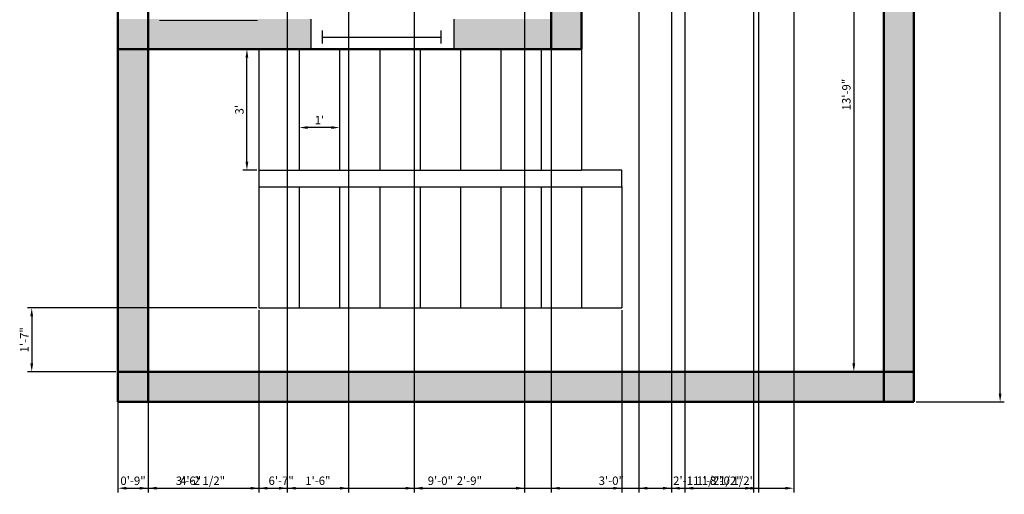
# Model space of a CAD drawing. Units: millimetres. Extents: x 2877 to 3173, y 802 to 1374.
# Tile 1 of 5: x 2879 to 3173, y 802 to 943. Entities that reach past the tile are written whole.
import ezdxf

# ---------------------------------------------------------------- set-up
doc = ezdxf.new("R2010")
doc.units = ezdxf.units.MM
for name, color, linetype, lineweight in [('A-WALL-PATT', 3, 'Continuous', 13), ('dimensions', 140, 'Continuous', 18), ('furniture', 70, 'Continuous', 18), ('staircase', 30, 'Continuous', 30), ('walls', 50, 'Continuous', 50), ('windows', 190, 'Continuous', 25)]:
    doc.layers.add(name, color=color, linetype=linetype, lineweight=lineweight)
doc.styles.get("Standard").update_dxf_attribs({"font": 'arial.ttf'})
doc.dimstyles.new('ISO-25', dxfattribs={"dimtxt": 2.5, "dimasz": 2.5, "dimexe": 1.25, "dimexo": 0.625, "dimtad": 1, "dimdec": 0, "dimlunit": 3, "dimtxsty": 'Standard', "dimcen": 2.5, "dimadec": 0, "dimazin": 0, "dimtfac": 1, "dimtdec": 0, "dimtmove": 0, "dimatfit": 3, "dimfxl": 1, "dimarcsym": 0})

# ---------------------------------------------------------------- blocks, each defined once
blk = doc.blocks.new('*U4')
for p, q in [((0, 4), (0, 0)), ((36, 4), (36, 0)), ((0, 2), (36, 2))]:
    blk.add_line(p, q)
blk = doc.blocks.new('*D20')
at = {"layer": 'Defpoints', "color": 0, "transparency": 16777216}
for p in [(3127.73, 1003.28), (3127.73, 838.28), (3127.73, 838.28)]:
    blk.add_point(p, dxfattribs=at)
at = {"layer": 'dimensions', "color": 0, "lineweight": -2, "transparency": 16777216}
for p, q in [((3128.35, 1003.28), (3128.98, 1003.28)), ((3127.73, 1000.78), (3127.73, 840.78)), ((3128.35, 838.28), (3128.98, 838.28))]:
    blk.add_line(p, q, dxfattribs=at)
at = {"layer": 'dimensions', "color": 0, "transparency": 16777216}
for points in [[(3127.31, 1000.78), (3128.14, 1000.78), (3127.73, 1003.28)], [(3127.31, 840.78), (3128.14, 840.78), (3127.73, 838.28)]]:
    blk.add_solid(points, dxfattribs=at)
at = {"layer": 'dimensions', "color": 0, "transparency": 16777216, "insert": (3125.83, 920.78), "char_height": 2.5, "attachment_point": 5, "rotation": 90}
blk.add_mtext('13\'-9"', dxfattribs=at)
blk = doc.blocks.new('*D21')
at = {"layer": 'Defpoints', "color": 0, "transparency": 16777216}
for p in [(2962.62, 913.6), (2974.62, 913.6), (2962.62, 910.97)]:
    blk.add_point(p, dxfattribs=at)
at = {"layer": 'dimensions', "color": 0, "lineweight": -2, "transparency": 16777216}
for p, q in [((2962.62, 912.98), (2962.62, 909.72)), ((2974.62, 912.98), (2974.62, 909.72)), ((2972.12, 910.97), (2965.12, 910.97))]:
    blk.add_line(p, q, dxfattribs=at)
at = {"layer": 'dimensions', "color": 0, "transparency": 16777216}
for points in [[(2965.12, 911.39), (2965.12, 910.55), (2962.62, 910.97)], [(2972.12, 911.39), (2972.12, 910.55), (2974.62, 910.97)]]:
    blk.add_solid(points, dxfattribs=at)
at = {"layer": 'dimensions', "color": 0, "transparency": 16777216, "insert": (2968.62, 912.85), "char_height": 2.5, "attachment_point": 5}
blk.add_mtext("1'", dxfattribs=at)
blk = doc.blocks.new('*D22')
at = {"layer": 'Defpoints', "color": 0, "transparency": 16777216}
for p in [(2947.03, 934.28), (2950.62, 934.28), (2950.62, 898.28)]:
    blk.add_point(p, dxfattribs=at)
at = {"layer": 'dimensions', "color": 0, "lineweight": -2, "transparency": 16777216}
for p, q in [((2950, 934.28), (2945.78, 934.28)), ((2947.03, 900.78), (2947.03, 931.78)), ((2950, 898.28), (2945.78, 898.28))]:
    blk.add_line(p, q, dxfattribs=at)
at = {"layer": 'dimensions', "color": 0, "transparency": 16777216}
for points in [[(2946.61, 931.78), (2947.44, 931.78), (2947.03, 934.28)], [(2946.61, 900.78), (2947.44, 900.78), (2947.03, 898.28)]]:
    blk.add_solid(points, dxfattribs=at)
at = {"layer": 'dimensions', "color": 0, "transparency": 16777216, "insert": (2945.12, 916.28), "char_height": 2.5, "attachment_point": 5, "rotation": 90}
blk.add_mtext("3'", dxfattribs=at)
blk = doc.blocks.new('*D35')
at = {"layer": 'Defpoints', "color": 0, "transparency": 16777216}
for p in [(3145.62, 1342.28), (3171.28, 1342.28), (3145.62, 829.28)]:
    blk.add_point(p, dxfattribs=at)
at = {"layer": 'dimensions', "color": 0, "lineweight": -2, "transparency": 16777216}
for p, q in [((3146.25, 1342.28), (3172.53, 1342.28)), ((3171.28, 831.78), (3171.28, 1339.78)), ((3146.25, 829.28), (3172.53, 829.28))]:
    blk.add_line(p, q, dxfattribs=at)
at = {"layer": 'dimensions', "color": 0, "transparency": 16777216}
for points in [[(3170.87, 1339.78), (3171.7, 1339.78), (3171.28, 1342.28)], [(3170.87, 831.78), (3171.7, 831.78), (3171.28, 829.28)]]:
    blk.add_solid(points, dxfattribs=at)
at = {"layer": 'dimensions', "color": 0, "transparency": 16777216, "insert": (3169.38, 1085.78), "char_height": 2.5, "attachment_point": 5, "rotation": 90}
blk.add_mtext('42\'-9"', dxfattribs=at)
blk = doc.blocks.new('*D36')
at = {"layer": 'Defpoints', "color": 0, "transparency": 16777216}
for p in [(2908.62, 1301.43), (2917.62, 1301.43), (2917.62, 803.61)]:
    blk.add_point(p, dxfattribs=at)
at = {"layer": 'dimensions', "color": 0, "lineweight": -2, "transparency": 16777216}
for p, q in [((2908.62, 1300.81), (2908.62, 802.36)), ((2917.62, 1300.81), (2917.62, 802.36)), ((2911.12, 803.61), (2915.12, 803.61))]:
    blk.add_line(p, q, dxfattribs=at)
at = {"layer": 'dimensions', "color": 0, "transparency": 16777216}
for points in [[(2911.12, 804.03), (2911.12, 803.2), (2908.62, 803.61)], [(2915.12, 804.03), (2915.12, 803.2), (2917.62, 803.61)]]:
    blk.add_solid(points, dxfattribs=at)
at = {"layer": 'dimensions', "color": 0, "transparency": 16777216, "insert": (2913.12, 805.52), "char_height": 2.5, "attachment_point": 5}
blk.add_mtext('0\'-9"', dxfattribs=at)
blk = doc.blocks.new('*D37')
at = {"layer": 'Defpoints', "color": 0, "transparency": 16777216}
for p in [(2950.62, 857.28), (3058.62, 857.28), (3058.62, 803.61)]:
    blk.add_point(p, dxfattribs=at)
at = {"layer": 'dimensions', "color": 0, "lineweight": -2, "transparency": 16777216}
for p, q in [((2950.62, 856.65), (2950.62, 802.36)), ((3058.62, 856.65), (3058.62, 802.36)), ((2953.12, 803.61), (3056.12, 803.61))]:
    blk.add_line(p, q, dxfattribs=at)
at = {"layer": 'dimensions', "color": 0, "transparency": 16777216}
for points in [[(2953.12, 804.03), (2953.12, 803.2), (2950.62, 803.61)], [(3056.12, 804.03), (3056.12, 803.2), (3058.62, 803.61)]]:
    blk.add_solid(points, dxfattribs=at)
at = {"layer": 'dimensions', "color": 0, "transparency": 16777216, "insert": (3004.62, 805.52), "char_height": 2.5, "attachment_point": 5}
blk.add_mtext('9\'-0"', dxfattribs=at)
blk = doc.blocks.new('*D38')
at = {"layer": 'Defpoints', "color": 0, "transparency": 16777216}
for p in [(2950.62, 857.28), (2908.62, 829.28), (2950.62, 803.61)]:
    blk.add_point(p, dxfattribs=at)
at = {"layer": 'dimensions', "color": 0, "lineweight": -2, "transparency": 16777216}
for p, q in [((2950.62, 856.65), (2950.62, 802.36)), ((2908.62, 828.65), (2908.62, 802.36)), ((2911.12, 803.61), (2948.12, 803.61))]:
    blk.add_line(p, q, dxfattribs=at)
at = {"layer": 'dimensions', "color": 0, "transparency": 16777216}
for points in [[(2911.12, 804.03), (2911.12, 803.2), (2908.62, 803.61)], [(2948.12, 804.03), (2948.12, 803.2), (2950.62, 803.61)]]:
    blk.add_solid(points, dxfattribs=at)
at = {"layer": 'dimensions', "color": 0, "transparency": 16777216, "insert": (2929.62, 805.52), "char_height": 2.5, "attachment_point": 5}
blk.add_mtext('3\'-6"', dxfattribs=at)
blk = doc.blocks.new('*D39')
at = {"layer": 'Defpoints', "color": 0, "transparency": 16777216}
for p in [(2950.62, 857.28), (2882.96, 838.28), (2908.62, 838.28)]:
    blk.add_point(p, dxfattribs=at)
at = {"layer": 'dimensions', "color": 0, "lineweight": -2, "transparency": 16777216}
for p, q in [((2950, 857.28), (2881.71, 857.28)), ((2882.96, 854.78), (2882.96, 840.78)), ((2908, 838.28), (2881.71, 838.28))]:
    blk.add_line(p, q, dxfattribs=at)
at = {"layer": 'dimensions', "color": 0, "transparency": 16777216}
for points in [[(2882.54, 854.78), (2883.38, 854.78), (2882.96, 857.28)], [(2882.54, 840.78), (2883.38, 840.78), (2882.96, 838.28)]]:
    blk.add_solid(points, dxfattribs=at)
at = {"layer": 'dimensions', "color": 0, "transparency": 16777216, "insert": (2881.08, 847.78), "char_height": 2.5, "attachment_point": 5, "rotation": 90}
blk.add_mtext('1\'-7"', dxfattribs=at)
blk = doc.blocks.new('*D40')
at = {"layer": 'Defpoints', "color": 0, "transparency": 16777216}
for p in [(3063.76, 1264.28), (3099.39, 1264.17), (3099.39, 803.61)]:
    blk.add_point(p, dxfattribs=at)
at = {"layer": 'dimensions', "color": 0, "lineweight": -2, "transparency": 16777216}
for p, q in [((3063.76, 1263.65), (3063.76, 802.36)), ((3099.39, 1263.55), (3099.39, 802.36)), ((3066.26, 803.61), (3096.89, 803.61))]:
    blk.add_line(p, q, dxfattribs=at)
at = {"layer": 'dimensions', "color": 0, "transparency": 16777216}
for points in [[(3066.26, 804.03), (3066.26, 803.2), (3063.76, 803.61)], [(3096.89, 804.03), (3096.89, 803.2), (3099.39, 803.61)]]:
    blk.add_solid(points, dxfattribs=at)
at = {"layer": 'dimensions', "color": 0, "transparency": 16777216, "insert": (3081.57, 805.53), "char_height": 2.5, "attachment_point": 5}
blk.add_mtext('2\'-11 1/2"', dxfattribs=at)
blk = doc.blocks.new('*D42')
at = {"layer": 'Defpoints', "color": 0, "transparency": 16777216}
for p in [(3073.41, 1003.28), (3109.83, 1003.28), (3109.83, 803.61)]:
    blk.add_point(p, dxfattribs=at)
at = {"layer": 'dimensions', "color": 0, "lineweight": -2, "transparency": 16777216}
for p, q in [((3073.41, 1002.65), (3073.41, 802.36)), ((3109.83, 1002.65), (3109.83, 802.36)), ((3075.91, 803.61), (3107.33, 803.61))]:
    blk.add_line(p, q, dxfattribs=at)
at = {"layer": 'dimensions', "color": 0, "transparency": 16777216}
for points in [[(3075.91, 804.03), (3075.91, 803.2), (3073.41, 803.61)], [(3107.33, 804.03), (3107.33, 803.2), (3109.83, 803.61)]]:
    blk.add_solid(points, dxfattribs=at)
at = {"layer": 'dimensions', "color": 0, "transparency": 16777216, "insert": (3091.62, 805.53), "char_height": 2.5, "attachment_point": 5}
blk.add_mtext('3\'-0 1/2"', dxfattribs=at)
blk = doc.blocks.new('*D43')
at = {"layer": 'Defpoints', "color": 0, "transparency": 16777216}
for p in [(3037.62, 1003.28), (3073.41, 1003.28), (3073.41, 803.61)]:
    blk.add_point(p, dxfattribs=at)
at = {"layer": 'dimensions', "color": 0, "lineweight": -2, "transparency": 16777216}
for p, q in [((3037.62, 1002.65), (3037.62, 802.36)), ((3073.41, 1002.65), (3073.41, 802.36)), ((3040.12, 803.61), (3070.91, 803.61))]:
    blk.add_line(p, q, dxfattribs=at)
at = {"layer": 'dimensions', "color": 0, "transparency": 16777216}
for points in [[(3040.12, 804.03), (3040.12, 803.2), (3037.62, 803.61)], [(3070.91, 804.03), (3070.91, 803.2), (3073.41, 803.61)]]:
    blk.add_solid(points, dxfattribs=at)
at = {"layer": 'dimensions', "color": 0, "transparency": 16777216, "insert": (3055.52, 805.52), "char_height": 2.5, "attachment_point": 5}
blk.add_mtext('3\'-0"', dxfattribs=at)
blk = doc.blocks.new('*D44')
at = {"layer": 'Defpoints', "color": 0, "transparency": 16777216}
for p in [(2996.81, 1237.82), (3029.69, 1237.82), (3029.69, 803.61)]:
    blk.add_point(p, dxfattribs=at)
at = {"layer": 'dimensions', "color": 0, "lineweight": -2, "transparency": 16777216}
for p, q in [((2996.81, 1237.19), (2996.81, 802.36)), ((3029.69, 1237.19), (3029.69, 802.36)), ((2999.31, 803.61), (3027.19, 803.61))]:
    blk.add_line(p, q, dxfattribs=at)
at = {"layer": 'dimensions', "color": 0, "transparency": 16777216}
for points in [[(2999.31, 804.03), (2999.31, 803.2), (2996.81, 803.61)], [(3027.19, 804.03), (3027.19, 803.2), (3029.69, 803.61)]]:
    blk.add_solid(points, dxfattribs=at)
at = {"layer": 'dimensions', "color": 0, "transparency": 16777216, "insert": (3013.25, 805.52), "char_height": 2.5, "attachment_point": 5}
blk.add_mtext('2\'-9"', dxfattribs=at)
blk = doc.blocks.new('*D46')
at = {"layer": 'Defpoints', "color": 0, "transparency": 16777216}
for p in [(2959.04, 1135.28), (2977.25, 1135.28), (2977.25, 803.61)]:
    blk.add_point(p, dxfattribs=at)
at = {"layer": 'dimensions', "color": 0, "lineweight": -2, "transparency": 16777216}
for p, q in [((2959.04, 1134.65), (2959.04, 802.36)), ((2977.25, 1134.65), (2977.25, 802.36)), ((2961.54, 803.61), (2974.75, 803.61))]:
    blk.add_line(p, q, dxfattribs=at)
at = {"layer": 'dimensions', "color": 0, "transparency": 16777216}
for points in [[(2961.54, 804.03), (2961.54, 803.2), (2959.04, 803.61)], [(2974.75, 804.03), (2974.75, 803.2), (2977.25, 803.61)]]:
    blk.add_solid(points, dxfattribs=at)
at = {"layer": 'dimensions', "color": 0, "transparency": 16777216, "insert": (2968.15, 805.52), "char_height": 2.5, "attachment_point": 5}
blk.add_mtext('1\'-6"', dxfattribs=at)
blk = doc.blocks.new('*D47')
at = {"layer": 'Defpoints', "color": 0, "transparency": 16777216}
for p in [(2908.62, 1135.28), (2959.04, 1135.28), (2959.04, 803.61)]:
    blk.add_point(p, dxfattribs=at)
at = {"layer": 'dimensions', "color": 0, "lineweight": -2, "transparency": 16777216}
for p, q in [((2908.62, 1134.65), (2908.62, 802.36)), ((2959.04, 1134.65), (2959.04, 802.36)), ((2911.12, 803.61), (2956.54, 803.61))]:
    blk.add_line(p, q, dxfattribs=at)
at = {"layer": 'dimensions', "color": 0, "transparency": 16777216}
for points in [[(2911.12, 804.03), (2911.12, 803.2), (2908.62, 803.61)], [(2956.54, 804.03), (2956.54, 803.2), (2959.04, 803.61)]]:
    blk.add_solid(points, dxfattribs=at)
at = {"layer": 'dimensions', "color": 0, "transparency": 16777216, "insert": (2933.83, 805.53), "char_height": 2.5, "attachment_point": 5}
blk.add_mtext('4\'-2 1/2"', dxfattribs=at)
blk = doc.blocks.new('*D64')
at = {"layer": 'Defpoints', "color": 0, "transparency": 16777216}
for p in [(3077.4, 1095.65), (3097.88, 1095.65), (3097.88, 803.61)]:
    blk.add_point(p, dxfattribs=at)
at = {"layer": 'dimensions', "color": 0, "lineweight": -2, "transparency": 16777216}
for p, q in [((3077.4, 1095.02), (3077.4, 802.36)), ((3097.88, 1095.02), (3097.88, 802.36)), ((3079.9, 803.61), (3095.38, 803.61))]:
    blk.add_line(p, q, dxfattribs=at)
at = {"layer": 'dimensions', "color": 0, "transparency": 16777216}
for points in [[(3079.9, 804.03), (3079.9, 803.2), (3077.4, 803.61)], [(3095.38, 804.03), (3095.38, 803.2), (3097.88, 803.61)]]:
    blk.add_solid(points, dxfattribs=at)
at = {"layer": 'dimensions', "color": 0, "transparency": 16777216, "insert": (3087.64, 805.53), "char_height": 2.5, "attachment_point": 5}
blk.add_mtext('1\'-8 1/2"', dxfattribs=at)
blk = doc.blocks.new('*D66')
at = {"layer": 'Defpoints', "color": 0, "transparency": 16777216}
for p in [(2917.62, 1257.52), (2996.81, 1237.82), (2996.81, 803.61)]:
    blk.add_point(p, dxfattribs=at)
at = {"layer": 'dimensions', "color": 0, "lineweight": -2, "transparency": 16777216}
for p, q in [((2917.62, 1256.89), (2917.62, 802.36)), ((2996.81, 1237.19), (2996.81, 802.36)), ((2920.12, 803.61), (2994.31, 803.61))]:
    blk.add_line(p, q, dxfattribs=at)
at = {"layer": 'dimensions', "color": 0, "transparency": 16777216}
for points in [[(2920.12, 804.03), (2920.12, 803.2), (2917.62, 803.61)], [(2994.31, 804.03), (2994.31, 803.2), (2996.81, 803.61)]]:
    blk.add_solid(points, dxfattribs=at)
at = {"layer": 'dimensions', "color": 0, "transparency": 16777216, "insert": (2957.22, 805.52), "char_height": 2.5, "attachment_point": 5}
blk.add_mtext('6\'-7"', dxfattribs=at)

msp = doc.modelspace()

# ---------------------------------------------------------------- hatches: boundary and pattern name
at = {"layer": 'A-WALL-PATT'}
h = msp.add_hatch(color=256, dxfattribs=at)
h.dxf.hatch_style = 1
h.paths.add_polyline_path([(3046.62, 1333.28), (3037.62, 1333.28), (3037.62, 1273.28), (3046.62, 1273.28)])
h.paths.add_polyline_path([(3046.62, 1273.28), (3037.62, 1273.28), (3037.62, 1264.28), (3046.62, 1264.28)])
h.paths.add_polyline_path([(3046.62, 1264.28), (3037.62, 1264.28), (3037.62, 1204.28), (3046.62, 1204.28)])
h.paths.add_polyline_path([(3136.62, 1273.28), (3099.39, 1273.28), (3099.39, 1264.28), (3136.62, 1264.28)])
h.paths.add_polyline_path([(3145.62, 1273.28), (3136.62, 1273.28), (3136.62, 1264.28), (3145.62, 1264.28)])
h.paths.add_polyline_path([(3145.62, 1264.28), (3136.62, 1264.28), (3136.62, 1198.76), (3145.62, 1198.76)])
h.paths.add_polyline_path([(3145.62, 1333.28), (3136.62, 1333.28), (3136.62, 1273.28), (3145.62, 1273.28)])
h.paths.add_polyline_path([(3145.62, 1342.28), (3136.62, 1342.28), (3136.62, 1333.28), (3145.62, 1333.28)])
h.paths.add_polyline_path([(3136.62, 1342.28), (3046.62, 1342.28), (3046.62, 1333.28), (3136.62, 1333.28)])
h.paths.add_polyline_path([(3046.62, 1342.28), (3037.62, 1342.28), (3037.62, 1333.28), (3046.62, 1333.28)])
h.paths.add_polyline_path([(2917.62, 1333.28), (2908.62, 1333.28), (2908.62, 1301.43), (2917.62, 1301.43)])
h.paths.add_polyline_path([(2917.62, 1257.52), (2908.62, 1257.52), (2908.62, 1213.28), (2917.62, 1213.28)])
h.paths.add_polyline_path([(2989.62, 1213.28), (2917.62, 1213.28), (2917.62, 1204.28), (2989.62, 1204.28)])
h.paths.add_polyline_path([(2998.62, 1213.28), (2989.62, 1213.28), (2989.62, 1204.28), (2998.62, 1204.28)])
h.paths.add_polyline_path([(2998.62, 1204.28), (2989.62, 1204.28), (2989.62, 1144.28), (2998.62, 1144.28)])
h.paths.add_polyline_path([(2998.62, 1144.28), (2989.62, 1144.28), (2989.62, 1135.28), (2998.62, 1135.28)])
h.paths.add_polyline_path([(2989.62, 1144.28), (2977.25, 1144.28), (2977.25, 1137.64), (2977.25, 1135.28), (2989.62, 1135.28)])
h.paths.add_polyline_path([(3006.77, 1141.79), (3006.77, 1144.28), (2998.62, 1144.28), (2998.62, 1135.28), (3007.71, 1135.28, -0.072018)])
h.paths.add_polyline_path([(3046.62, 1135.28), (3037.62, 1135.28), (3037.62, 1012.28), (3046.62, 1012.28)])
h.paths.add_polyline_path([(3046.62, 1144.28), (3037.62, 1144.28), (3037.62, 1135.28), (3046.62, 1135.28)])
h.paths.add_polyline_path([(3037.62, 1144.28), (3029.73, 1144.28), (3029.73, 1141.79), (3029.73, 1135.28), (3037.62, 1135.28)])
h.paths.add_polyline_path([(3145.62, 1158.87), (3136.62, 1158.87), (3136.62, 1012.28), (3145.62, 1012.28)])
h.paths.add_polyline_path([(3145.62, 1003.28), (3136.62, 1003.28), (3136.62, 838.28), (3145.62, 838.28)])
h.paths.add_polyline_path([(3145.62, 1012.28), (3136.62, 1012.28), (3136.62, 1003.28), (3145.62, 1003.28)])
h.paths.add_polyline_path([(3136.62, 1012.28), (3109.83, 1012.28), (3109.83, 1006.01), (3109.83, 1003.28), (3136.62, 1003.28)])
h.paths.add_polyline_path([(3073.41, 1012.28), (3046.62, 1012.28), (3046.62, 1003.28), (3073.41, 1003.28), (3073.41, 1006.01)])
h.paths.add_polyline_path([(3046.62, 1012.28), (3037.62, 1012.28), (3037.62, 1003.28), (3046.62, 1003.28)])
h.paths.add_polyline_path([(3046.62, 1003.28), (3037.62, 1003.28), (3037.62, 943.28), (3046.62, 943.28)])
h.paths.add_polyline_path([(3136.62, 838.28), (2917.62, 838.28), (2917.62, 829.28), (3136.62, 829.28)])
h.paths.add_polyline_path([(3145.62, 838.28), (3136.62, 838.28), (3136.62, 829.28), (3145.62, 829.28)])
h.paths.add_polyline_path([(2917.62, 934.28), (2908.62, 934.28), (2908.62, 838.28), (2917.62, 838.28)])
h.paths.add_polyline_path([(2917.62, 838.28), (2908.62, 838.28), (2908.62, 829.28), (2917.62, 829.28)])
h.paths.add_polyline_path([(2917.62, 943.28), (2908.62, 943.28), (2908.62, 934.28), (2917.62, 934.28)])
h.paths.add_polyline_path([(2966.07, 943.28), (2917.62, 943.28), (2917.62, 934.28), (2966.07, 934.28)])
h.paths.add_polyline_path([(3046.62, 943.28), (3037.62, 943.28), (3037.62, 934.28), (3046.62, 934.28)])
h.paths.add_polyline_path([(3037.62, 943.28), (3008.74, 943.28), (3008.74, 934.28), (3037.62, 934.28)])

# ---------------------------------------------------------------- linework, layer by layer
at = {"layer": 'furniture'}
msp.add_line((2921, 942.88), (2950.14, 942.88), dxfattribs=at)
at = {"layer": 'staircase'}
for p, q in [((2950.62, 934.28), (2950.62, 898.28)), ((2962.62, 934.28), (2962.62, 898.28)), ((2974.62, 934.28), (2974.62, 898.28)), ((2986.62, 934.28), (2986.62, 898.28)), ((2998.62, 934.28), (2998.62, 898.28)), ((3010.62, 934.28), (3010.62, 898.28)), ((3022.62, 934.28), (3022.62, 898.28)), ((3034.62, 934.28), (3034.62, 898.28)), ((3046.62, 934.28), (3046.62, 898.28)), ((2950.62, 898.28), (3046.62, 898.28)), ((2950.62, 898.28), (2950.62, 893.28)), ((3057.46, 898.28), (3046.62, 898.28)), ((3058.62, 898.28), (3057.47, 898.28)), ((3058.62, 893.28), (3058.62, 898.28)), ((2950.62, 893.28), (3058.62, 893.28)), ((2950.62, 893.28), (2950.62, 857.28)), ((2962.62, 893.28), (2962.62, 857.28)), ((2974.62, 893.28), (2974.62, 857.28)), ((2986.62, 893.28), (2986.62, 857.28)), ((2998.62, 893.28), (2998.62, 857.28)), ((3010.62, 893.28), (3010.62, 857.28)), ((3022.62, 893.28), (3022.62, 857.28)), ((3034.62, 893.28), (3034.62, 857.28)), ((3046.62, 893.28), (3046.62, 857.28)), ((3058.62, 893.28), (3058.62, 857.28)), ((2950.62, 857.28), (3058.62, 857.28))]:
    msp.add_line(p, q, dxfattribs=at)
at = {"layer": 'walls'}
for p, q in [((2908.62, 1342.28), (2908.62, 829.28)), ((2917.62, 1342.28), (2917.62, 829.28)), ((3136.62, 1342.28), (3136.62, 829.28)), ((3145.62, 1342.28), (3145.62, 829.28)), ((3037.62, 1144.28), (3037.62, 934.28)), ((3046.62, 1144.28), (3046.62, 934.28)), ((2908.62, 934.28), (3046.62, 934.28)), ((2908.62, 838.28), (3145.62, 838.28)), ((2908.62, 829.28), (3145.62, 829.28))]:
    msp.add_line(p, q, dxfattribs=at)
at = {"layer": 'windows'}
for p, q in [((2966.07, 943.28), (2966.07, 934.28)), ((3008.74, 934.28), (3008.74, 943.28))]:
    msp.add_line(p, q, dxfattribs=at)

# ---------------------------------------------------------------- block references
at = {"layer": 'windows', "xscale": 0.9804508946843826, "yscale": 0.9804508946843826, "zscale": 0.9804508946843826}
msp.add_blockref('*U4', (2969.43, 935.95), dxfattribs=at)

# ---------------------------------------------------------------- dimensions: what is measured, and where the dimension line sits
at = {"layer": 'dimensions'}
for base, p1, p2, override, picture, middle in [((3171.28, 1342.28), (3145.62, 829.28), (3145.62, 1342.28), {"dimdec": 1, "dimlfac": 1, "dimrnd": 0, "dimzin": 1, "dimdsep": 46, "dimlunit": 4, "dimfrac": 2}, '*D35', (3169.38, 1085.78)), ((3127.73, 838.28), (3127.73, 1003.28), (3127.73, 838.28), {"dimclrd": 0, "dimclre": 0, "dimclrt": 0}, '*D20', (3125.83, 920.78)), ((2947.03, 934.28), (2950.62, 898.28), (2950.62, 934.28), {"dimclrd": 0, "dimclre": 0, "dimclrt": 0}, '*D22', (2945.12, 916.28)), ((2882.96, 838.28), (2950.62, 857.28), (2908.62, 838.28), {"dimdec": 1, "dimlfac": 1, "dimrnd": 0, "dimzin": 1, "dimdsep": 46, "dimlunit": 4, "dimfrac": 2}, '*D39', (2881.08, 847.78))]:
    dim = msp.add_linear_dim(base=base, p1=p1, p2=p2, angle=90, dimstyle='ISO-25', override=override, dxfattribs=at)
    dim.commit()
    dim.dimension.update_dxf_attribs({"geometry": picture, "text_midpoint": middle})
for base, p1, p2, override, picture, middle in [((2917.62, 803.61), (2908.62, 1301.43), (2917.62, 1301.43), {"dimdec": 1, "dimlfac": 1, "dimrnd": 0, "dimzin": 1, "dimdsep": 46, "dimlunit": 4, "dimfrac": 2}, '*D36', (2913.12, 805.52)), ((3099.39, 803.61), (3063.76, 1264.28), (3099.39, 1264.17), {"dimdec": 1, "dimlfac": 1, "dimrnd": 0, "dimzin": 1, "dimdsep": 46, "dimlunit": 4, "dimfrac": 2}, '*D40', (3081.57, 805.53)), ((2996.81, 803.61), (2917.62, 1257.52), (2996.81, 1237.82), {"dimdec": 1, "dimlfac": 1, "dimrnd": 0, "dimzin": 1, "dimdsep": 46, "dimlunit": 4, "dimfrac": 2}, '*D66', (2957.22, 805.52)), ((3029.69, 803.61), (2996.81, 1237.82), (3029.69, 1237.82), {"dimdec": 1, "dimlfac": 1, "dimrnd": 0, "dimzin": 1, "dimdsep": 46, "dimlunit": 4, "dimfrac": 2}, '*D44', (3013.25, 805.52)), ((2959.04, 803.61), (2908.62, 1135.28), (2959.04, 1135.28), {"dimdec": 1, "dimlfac": 1, "dimrnd": 0, "dimzin": 1, "dimdsep": 46, "dimlunit": 4, "dimfrac": 2}, '*D47', (2933.83, 805.53)), ((2977.25, 803.61), (2959.04, 1135.28), (2977.25, 1135.28), {"dimdec": 1, "dimlfac": 1, "dimrnd": 0, "dimzin": 1, "dimdsep": 46, "dimlunit": 4, "dimfrac": 2}, '*D46', (2968.15, 805.52)), ((3097.88, 803.61), (3077.4, 1095.65), (3097.88, 1095.65), {"dimdec": 1, "dimlfac": 1, "dimrnd": 0, "dimzin": 1, "dimdsep": 46, "dimlunit": 4, "dimfrac": 2}, '*D64', (3087.64, 805.53)), ((3073.41, 803.61), (3037.62, 1003.28), (3073.41, 1003.28), {"dimdec": 1, "dimlfac": 1, "dimrnd": 0, "dimzin": 1, "dimdsep": 46, "dimlunit": 4, "dimfrac": 2}, '*D43', (3055.52, 805.52)), ((3109.83, 803.61), (3073.41, 1003.28), (3109.83, 1003.28), {"dimdec": 1, "dimlfac": 1, "dimrnd": 0, "dimzin": 1, "dimdsep": 46, "dimlunit": 4, "dimfrac": 2}, '*D42', (3091.62, 805.53)), ((2962.62, 910.97), (2974.62, 913.6), (2962.62, 913.6), {"dimclrd": 0, "dimclre": 0, "dimclrt": 0}, '*D21', (2968.62, 912.85)), ((2950.62, 803.61), (2908.62, 829.28), (2950.62, 857.28), {"dimdec": 1, "dimlfac": 1, "dimrnd": 0, "dimzin": 1, "dimdsep": 46, "dimlunit": 4, "dimfrac": 2}, '*D38', (2929.62, 805.52)), ((3058.62, 803.61), (2950.62, 857.28), (3058.62, 857.28), {"dimdec": 1, "dimlfac": 1, "dimrnd": 0, "dimzin": 1, "dimdsep": 46, "dimlunit": 4, "dimfrac": 2}, '*D37', (3004.62, 805.52))]:
    dim = msp.add_linear_dim(base=base, p1=p1, p2=p2, dimstyle='ISO-25', override=override, dxfattribs=at)
    dim.commit()
    dim.dimension.update_dxf_attribs({"geometry": picture, "text_midpoint": middle})

doc.saveas('drawing.dxf')
